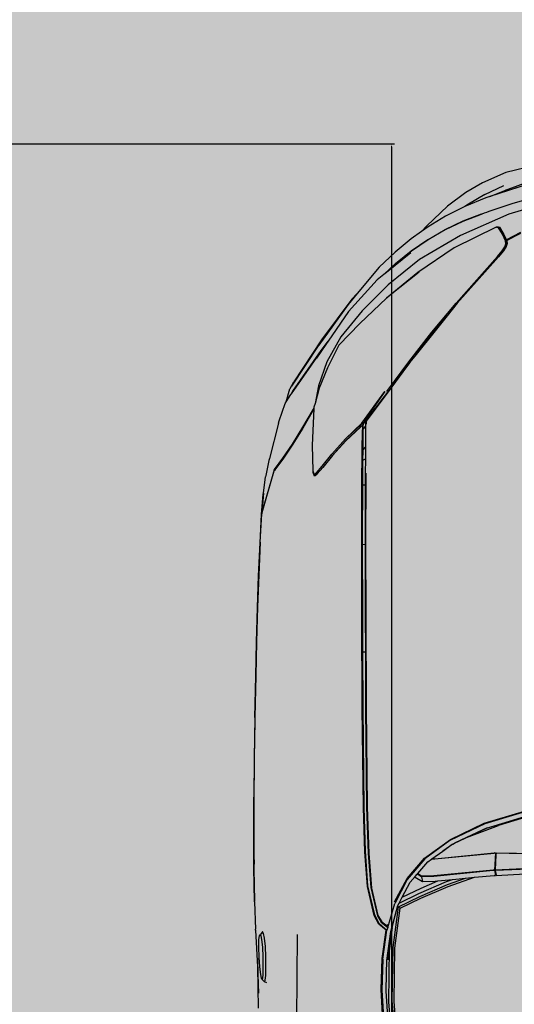
# Model space of a CAD drawing. Units: inches. Extents: x 1884 to 2398, y 474 to 1488.
# Tile 27 of 39: x 2275 to 2306, y 699 to 761. Entities that reach past the tile are written whole.
import ezdxf

# ---------------------------------------------------------------- set-up
doc = ezdxf.new("R2010")
doc.units = ezdxf.units.IN
doc.header["$MEASUREMENT"] = 0
doc.layers.get('0').update_dxf_attribs({"color": 250})
doc.layers.add('A-ANNO-DIMS', color=2, linetype='Continuous', lineweight=18)
doc.layers.add('C-VEHI', color=8, linetype='Continuous', lineweight=18)
doc.layers.add('Edges', color=250, linetype='Continuous')
doc.layers.add('L-PVMT-PATT', color=9, linetype='Continuous', lineweight=13, true_color=0xc7c8ca)
doc.styles.get("Standard").update_dxf_attribs({"font": 'arial.ttf'})
doc.dimstyles.get("Standard").update_dxf_attribs({"dimtxt": 7, "dimasz": 0.18, "dimexe": 0.18, "dimexo": 0.0625, "dimgap": 0.09, "dimtad": 0, "dimtih": 1, "dimtoh": 1, "dimzin": 0, "dimdsep": 46, "dimlunit": 3, "dimtxsty": 'Standard', "dimcen": 0.09, "dimadec": 0, "dimazin": 0, "dimtfac": 1, "dimtofl": 0, "dimtmove": 0, "dimatfit": 3, "dimfxl": 1, "dimtolj": 1, "dimtzin": 0, "dimarcsym": 0})

# ---------------------------------------------------------------- blocks, each defined once
blk = doc.blocks.new('Nissan Qashqai pl')
at = {"layer": 'Edges'}
for p, q in [((8.4086, 11.6764), (8.4045, 11.4011)), ((8.4305, 11.3996), (8.419, 11.6758)), ((8.4204, 11.6758), (8.4319, 11.3996)), ((8.4394, 11.4014), (8.4238, 11.6766)), ((7.3676, 11.5172), (7.3963, 11.4215)), ((7.3193, 11.4645), (7.3309, 11.4166)), ((8.3573, 11.3824), (8.3296, 11.4739)), ((8.3311, 11.4733), (8.3582, 11.3836)), ((8.3648, 11.3863), (8.3377, 11.4753)), ((8.3392, 11.4758), (8.3608, 11.4048)), ((7.344, 11.4572), (7.3596, 11.4139)), ((7.3467, 11.4596), (7.3686, 11.3913)), ((7.3489, 11.4517), (7.3686, 11.3913)), ((7.375, 11.4442), (7.3799, 11.4278)), ((7.4255, 11.4398), (7.4367, 11.4174)), ((7.4379, 11.4179), (7.4267, 11.4401)), ((8.4041, 11.4013), (8.4048, 11.4423)), ((7.3309, 11.4166), (7.347, 11.3798)), ((7.3799, 11.4278), (7.3845, 11.4136)), ((7.3963, 11.4215), (7.4302, 11.3449)), ((7.4387, 11.4162), (7.4282, 11.4113)), ((7.4283, 11.4135), (7.4359, 11.417)), ((7.4296, 11.4129), (7.4383, 11.417)), ((7.4359, 11.417), (7.4367, 11.4174)), ((7.4383, 11.417), (7.4367, 11.4174)), ((7.4375, 11.42), (7.4384, 11.4182)), ((7.4379, 11.4179), (7.4384, 11.4182)), ((7.4389, 11.4173), (7.4379, 11.4179)), ((7.4383, 11.417), (7.4379, 11.4179)), ((7.4389, 11.4173), (7.4383, 11.417)), ((7.4384, 11.4182), (7.4387, 11.4183)), ((7.4387, 11.4183), (7.443, 11.4188)), ((7.4431, 11.4166), (7.4387, 11.4162)), ((7.4389, 11.4173), (7.44, 11.4178)), ((7.4442, 11.4183), (7.44, 11.4178)), ((7.443, 11.4188), (7.4477, 11.4172)), ((7.4479, 11.4149), (7.4431, 11.4166)), ((7.4477, 11.4172), (7.4442, 11.4183)), ((7.4477, 11.4172), (7.4541, 11.4128)), ((7.3655, 11.3837), (7.3514, 11.4133)), ((7.3686, 11.3913), (7.3596, 11.4139)), ((7.3845, 11.4136), (7.3925, 11.3899)), ((7.4167, 11.4049), (7.417, 11.4065)), ((7.4172, 11.4047), (7.4167, 11.4049)), ((7.4169, 11.4036), (7.4167, 11.4049)), ((7.4282, 11.4113), (7.4169, 11.4044)), ((7.4172, 11.4047), (7.4169, 11.4044)), ((7.4169, 11.4044), (7.4169, 11.4036)), ((7.4172, 11.4018), (7.4169, 11.4036)), ((7.4169, 11.4036), (7.4169, 11.403)), ((7.4169, 11.403), (7.4172, 11.4011)), ((7.417, 11.4065), (7.4283, 11.4135)), ((7.4183, 11.406), (7.4172, 11.4047)), ((7.4174, 11.4013), (7.4172, 11.4018)), ((7.4172, 11.4011), (7.4498, 11.3349)), ((7.4174, 11.4013), (7.4175, 11.4012)), ((7.4296, 11.4129), (7.4183, 11.406)), ((7.4541, 11.4108), (7.4479, 11.4149)), ((7.4541, 11.4128), (7.4638, 11.4051)), ((7.4635, 11.4034), (7.4541, 11.4108)), ((7.5369, 11.3385), (7.4635, 11.4034)), ((7.4638, 11.4051), (7.5371, 11.34)), ((8.3799, 11.3545), (8.3608, 11.4048)), ((8.407, 11.401), (8.4037, 11.4002)), ((8.4037, 11.4002), (8.4314, 11.3985)), ((8.4037, 11.3992), (8.4037, 11.4002)), ((8.4041, 11.4013), (8.4045, 11.4011)), ((8.4045, 11.4011), (8.407, 11.401)), ((8.407, 11.401), (8.4305, 11.3996)), ((8.4314, 11.3985), (8.4394, 11.4004)), ((8.4319, 11.3996), (8.436, 11.4006)), ((8.436, 11.4006), (8.4394, 11.4014)), ((8.4394, 11.4004), (8.436, 11.4006)), ((8.4394, 11.3984), (8.4394, 11.4004)), ((7.3686, 11.3913), (7.3707, 11.3849)), ((7.3707, 11.3849), (7.3843, 11.3522)), ((7.3925, 11.3899), (7.3938, 11.3859)), ((7.3938, 11.3859), (7.3951, 11.3822)), ((8.3646, 11.387), (8.3799, 11.3545)), ((8.3888, 11.3355), (8.3648, 11.3863)), ((8.4037, 11.3992), (8.4046, 11.3981)), ((8.4042, 11.3983), (8.4037, 11.3992)), ((8.4134, 11.3049), (8.4042, 11.3983)), ((8.4046, 11.3981), (8.4138, 11.3048)), ((8.4305, 11.3996), (8.4319, 11.3996)), ((8.4306, 11.3966), (8.4314, 11.3975)), ((8.4398, 11.3032), (8.4306, 11.3966)), ((8.4314, 11.3985), (8.4314, 11.3975)), ((8.4314, 11.3975), (8.4319, 11.3967)), ((8.4319, 11.3967), (8.4412, 11.3033)), ((8.4425, 11.3672), (8.4394, 11.3984)), ((7.347, 11.3798), (7.3624, 11.3535)), ((7.3655, 11.3837), (7.3805, 11.3576)), ((7.3951, 11.3822), (7.3965, 11.3787)), ((7.3962, 11.3781), (7.3965, 11.3787)), ((7.4071, 11.3493), (7.3962, 11.3781)), ((7.3965, 11.3787), (7.3969, 11.3777)), ((7.3969, 11.3777), (7.4078, 11.349)), ((8.3826, 11.3291), (8.3573, 11.3824)), ((8.3582, 11.3836), (8.3844, 11.3284)), ((7.3624, 11.3535), (7.3837, 11.3245)), ((7.3805, 11.3576), (7.3843, 11.3522)), ((8.3799, 11.3545), (8.3888, 11.3355)), ((8.4571, 11.3258), (8.4425, 11.3672)), ((8.4439, 11.3531), (8.4425, 11.3672)), ((8.454, 11.3245), (8.4439, 11.3531)), ((8.4459, 11.3326), (8.4439, 11.3531)), ((7.3843, 11.3522), (7.3845, 11.3517)), ((7.3845, 11.3517), (7.3997, 11.3215)), ((7.4205, 11.3212), (7.4071, 11.3493)), ((7.4078, 11.349), (7.4211, 11.321)), ((7.4302, 11.3449), (7.4679, 11.2807)), ((7.5827, 11.3001), (7.5369, 11.3385)), ((7.5371, 11.34), (7.5568, 11.324)), ((7.3837, 11.3245), (7.4147, 11.2918)), ((7.4498, 11.3349), (7.4884, 11.2778)), ((7.584, 11.3013), (7.5568, 11.324)), ((7.5568, 11.324), (7.5829, 11.303)), ((8.4122, 11.2883), (8.3826, 11.3291)), ((8.3844, 11.3284), (8.4134, 11.2888)), ((8.3901, 11.3328), (8.3888, 11.3355)), ((8.3901, 11.3328), (8.4011, 11.3173)), ((8.3904, 11.3321), (8.3901, 11.3328)), ((8.4011, 11.3173), (8.3904, 11.3321)), ((8.4493, 11.3229), (8.4459, 11.3326)), ((8.4482, 11.3095), (8.4459, 11.3326)), ((8.468, 11.2793), (8.4493, 11.3229)), ((8.4725, 11.2812), (8.454, 11.3245)), ((8.4756, 11.2826), (8.4571, 11.3258)), ((7.3997, 11.3215), (7.4166, 11.2939)), ((7.4363, 11.294), (7.4205, 11.3212)), ((7.4211, 11.321), (7.4369, 11.2938)), ((8.4135, 11.3), (8.4011, 11.3173)), ((8.4594, 11.2831), (8.4482, 11.3095)), ((8.4487, 11.305), (8.4482, 11.3095)), ((7.4147, 11.2918), (7.4239, 11.2837)), ((7.4166, 11.2939), (7.4239, 11.2837)), ((7.4542, 11.2677), (7.4363, 11.294)), ((7.4369, 11.2938), (7.4549, 11.2675)), ((7.6296, 11.2639), (7.5827, 11.3001)), ((7.5829, 11.303), (7.618, 11.275)), ((7.618, 11.275), (7.584, 11.3013)), ((8.4135, 11.3), (8.4134, 11.3049)), ((8.4139, 11.2994), (8.4135, 11.3)), ((8.4138, 11.3048), (8.4139, 11.2994)), ((8.4183, 11.2934), (8.4139, 11.2994)), ((8.4365, 11.2776), (8.4183, 11.2934)), ((8.44, 11.2834), (8.4398, 11.3032)), ((8.4412, 11.3033), (8.4415, 11.2835)), ((8.4489, 11.2852), (8.4487, 11.305)), ((7.4239, 11.2837), (7.4354, 11.2675)), ((7.4679, 11.2807), (7.5081, 11.2311)), ((7.4882, 11.2797), (7.5243, 11.2341)), ((7.4884, 11.2778), (7.5289, 11.2283)), ((8.4444, 11.2608), (8.4122, 11.2883)), ((8.4134, 11.2888), (8.4462, 11.2609)), ((8.4365, 11.2776), (8.44, 11.2834)), ((8.4375, 11.2767), (8.4365, 11.2776)), ((8.4415, 11.2835), (8.4375, 11.2767)), ((8.4412, 11.2735), (8.4375, 11.2767)), ((8.4415, 11.2835), (8.4489, 11.2852)), ((8.4422, 11.2737), (8.4489, 11.2852)), ((8.4737, 11.2534), (8.4594, 11.2831)), ((8.4831, 11.2484), (8.468, 11.2793)), ((8.4889, 11.2473), (8.4725, 11.2812)), ((8.4914, 11.25), (8.4756, 11.2826)), ((7.4354, 11.2675), (7.4565, 11.2419)), ((7.4744, 11.2427), (7.4542, 11.2677)), ((7.4549, 11.2675), (7.475, 11.2426)), ((7.4574, 11.267), (7.4885, 11.2283)), ((7.618, 11.275), (7.6301, 11.2654)), ((7.676, 11.2289), (7.6296, 11.2639)), ((7.6301, 11.2654), (7.6306, 11.2651)), ((7.6306, 11.2651), (7.6306, 11.265)), ((7.6306, 11.265), (7.6373, 11.2601)), ((7.6373, 11.2601), (7.6769, 11.2312)), ((8.4422, 11.2737), (8.4412, 11.2735)), ((8.4499, 11.2659), (8.4412, 11.2735)), ((8.4814, 11.2413), (8.4444, 11.2608)), ((8.4462, 11.2609), (8.4838, 11.2415)), ((8.4737, 11.2534), (8.4499, 11.2659)), ((8.4831, 11.2484), (8.4737, 11.2534)), ((8.4867, 11.2465), (8.4831, 11.2484)), ((8.528, 11.2354), (8.4867, 11.2465)), ((8.5214, 11.2374), (8.4867, 11.2465)), ((8.4889, 11.2473), (8.4914, 11.25)), ((8.5531, 11.2387), (8.4889, 11.2473)), ((8.5544, 11.2416), (8.4914, 11.25)), ((8.7481, 11.2473), (8.6375, 11.2376)), ((8.7491, 11.2501), (8.6386, 11.2404)), ((7.4565, 11.2419), (7.4801, 11.2168)), ((7.4918, 11.2242), (7.4744, 11.2427)), ((7.475, 11.2426), (7.477, 11.2404)), ((7.477, 11.2404), (7.4765, 11.2411)), ((7.477, 11.2405), (7.4775, 11.2399)), ((7.4784, 11.2388), (7.477, 11.2404)), ((7.477, 11.2404), (7.4775, 11.2399)), ((7.4775, 11.2399), (7.4787, 11.2385)), ((7.4775, 11.2399), (7.4787, 11.2387)), ((7.4787, 11.2387), (7.4782, 11.2392)), ((7.4795, 11.2377), (7.4787, 11.2387)), ((7.4787, 11.2387), (7.4885, 11.2283)), ((7.5081, 11.2311), (7.5492, 11.1902)), ((7.5243, 11.2341), (7.5286, 11.2296)), ((7.6769, 11.2312), (7.7194, 11.1992)), ((7.7232, 11.1955), (7.6771, 11.2307)), ((8.5216, 11.2303), (8.4838, 11.2415)), ((8.5132, 11.2202), (8.5216, 11.2303)), ((8.5155, 11.2168), (8.5258, 11.2291)), ((8.5197, 11.2297), (8.5166, 11.2307)), ((8.5177, 11.2272), (8.5197, 11.2297)), ((8.5216, 11.2303), (8.5197, 11.2297)), ((8.5214, 11.2374), (8.555, 11.233)), ((8.5301, 11.2352), (8.5214, 11.2374)), ((8.5216, 11.2303), (8.5258, 11.2291)), ((8.5258, 11.2291), (8.5259, 11.2279)), ((8.5715, 11.2227), (8.5258, 11.2291)), ((8.5736, 11.2291), (8.528, 11.2354)), ((8.6375, 11.2376), (8.5531, 11.2387)), ((8.6386, 11.2404), (8.5544, 11.2416)), ((8.6387, 11.2319), (8.555, 11.233)), ((8.555, 11.233), (8.5726, 11.2307)), ((8.5941, 11.2286), (8.5736, 11.2291)), ((8.5941, 11.2289), (8.5941, 11.2286)), ((8.6699, 11.231), (8.622, 11.228)), ((8.6721, 11.2348), (8.6387, 11.2319)), ((7.4801, 11.2168), (7.5217, 11.1823)), ((7.4885, 11.2283), (7.4918, 11.2242)), ((7.4918, 11.2242), (7.5001, 11.2139)), ((7.5001, 11.2139), (7.5501, 11.1684)), ((7.5289, 11.2283), (7.5687, 11.1862)), ((7.7261, 11.1898), (7.6762, 11.2256)), ((7.6762, 11.2256), (7.7233, 11.1928)), ((8.4588, 11.2036), (8.5032, 11.2141)), ((8.4595, 11.2047), (8.5025, 11.2148)), ((8.5155, 11.2168), (8.5018, 11.2098)), ((8.5025, 11.2148), (8.5125, 11.221)), ((8.5163, 11.2162), (8.5029, 11.2092)), ((8.5032, 11.2141), (8.5132, 11.2202)), ((8.5125, 11.221), (8.5177, 11.2272)), ((8.5237, 11.2252), (8.5163, 11.2162)), ((8.5259, 11.2279), (8.5237, 11.2252)), ((8.5294, 11.2274), (8.5259, 11.2279)), ((8.5706, 11.2216), (8.5294, 11.2274)), ((8.6197, 11.2201), (8.5706, 11.2216)), ((8.5715, 11.2227), (8.6203, 11.2213)), ((8.622, 11.228), (8.5941, 11.2286)), ((8.6683, 11.2226), (8.6197, 11.2201)), ((8.6203, 11.2213), (8.6721, 11.2241)), ((7.7194, 11.1992), (7.7232, 11.1966)), ((8.1753, 11.1963), (8.3318, 11.198)), ((8.3318, 11.198), (8.4049, 11.2004)), ((8.332, 11.1971), (8.4042, 11.1995)), ((8.4559, 11.1991), (8.4014, 11.1953)), ((8.4571, 11.1983), (8.4022, 11.1943)), ((8.4042, 11.1995), (8.4588, 11.2036)), ((8.4049, 11.2004), (8.4595, 11.2047)), ((8.5018, 11.2098), (8.4559, 11.1991)), ((8.5029, 11.2092), (8.4571, 11.1983)), ((7.5304, 11.1737), (7.5217, 11.1823)), ((7.5217, 11.1823), (7.5387, 11.1682)), ((7.5492, 11.1902), (7.59, 11.1565)), ((7.5687, 11.1862), (7.6032, 11.1533)), ((7.7232, 11.1966), (7.7279, 11.1965)), ((7.7281, 11.1918), (7.7232, 11.1955)), ((7.7232, 11.1955), (7.7245, 11.1955)), ((7.7267, 11.1902), (7.7233, 11.1928)), ((7.7247, 11.1954), (7.7245, 11.1955)), ((7.7245, 11.1955), (7.7294, 11.1955)), ((7.7261, 11.1898), (7.7507, 11.1638)), ((7.7286, 11.1881), (7.7267, 11.1902)), ((7.7281, 11.1918), (7.7299, 11.1904)), ((7.7349, 11.1917), (7.7281, 11.1918)), ((7.753, 11.1648), (7.7281, 11.1918)), ((7.7507, 11.1638), (7.7286, 11.1881)), ((7.7294, 11.1955), (7.731, 11.1955)), ((7.7299, 11.1904), (7.7324, 11.1876)), ((7.7299, 11.1904), (7.7364, 11.1904)), ((7.731, 11.1955), (7.7349, 11.1917)), ((7.731, 11.1955), (7.764, 11.1953)), ((7.7324, 11.1876), (7.7539, 11.1642)), ((7.768, 11.1915), (7.7349, 11.1917)), ((7.7363, 11.1904), (7.7364, 11.1904)), ((7.7694, 11.1901), (7.7364, 11.1904)), ((7.764, 11.1953), (7.7636, 11.1957)), ((7.768, 11.1915), (7.764, 11.1953)), ((7.764, 11.1953), (7.7662, 11.1953)), ((7.7659, 11.1957), (7.7662, 11.1953)), ((7.7662, 11.1953), (7.7668, 11.1946)), ((7.7662, 11.1953), (7.7811, 11.1952)), ((7.7692, 11.1915), (7.768, 11.1915)), ((7.7694, 11.1901), (7.7687, 11.1908)), ((7.7844, 11.1913), (7.7692, 11.1915)), ((7.7707, 11.1901), (7.7694, 11.1901)), ((7.7851, 11.19), (7.7707, 11.1901)), ((7.7811, 11.1952), (7.7809, 11.1958)), ((7.7814, 11.1946), (7.7811, 11.1952)), ((7.7811, 11.1952), (7.7822, 11.1952)), ((7.7822, 11.1952), (7.7819, 11.1958)), ((7.7822, 11.1952), (7.8057, 11.195)), ((7.7844, 11.1913), (7.7822, 11.1952)), ((7.8078, 11.1911), (7.7844, 11.1913)), ((7.7846, 11.1909), (7.7851, 11.19)), ((7.8083, 11.1898), (7.7851, 11.19)), ((7.8048, 11.1959), (7.8233, 11.1958)), ((7.8057, 11.195), (7.8233, 11.195)), ((7.8233, 11.1911), (7.8078, 11.1911)), ((7.904, 11.1894), (7.8083, 11.1898)), ((7.8233, 11.195), (7.8233, 11.1958)), ((7.8233, 11.1958), (7.9014, 11.1955)), ((7.8233, 11.195), (7.902, 11.1947)), ((7.8233, 11.1911), (7.8233, 11.195)), ((7.8233, 11.1899), (7.8233, 11.1911)), ((7.9036, 11.1907), (7.8233, 11.1911)), ((7.9014, 11.1955), (7.9185, 11.1955)), ((7.902, 11.1947), (7.9183, 11.1947)), ((7.9176, 11.1908), (7.9036, 11.1907)), ((8.0276, 11.1896), (7.904, 11.1894)), ((7.9183, 11.1947), (7.9176, 11.1908)), ((8.0275, 11.1909), (7.9176, 11.1908)), ((7.9185, 11.1955), (7.9183, 11.1947)), ((7.9183, 11.1947), (8.0275, 11.1948)), ((7.9185, 11.1955), (8.0273, 11.1957)), ((8.0273, 11.1957), (8.1753, 11.1963)), ((8.0275, 11.1948), (8.0876, 11.1951)), ((8.0873, 11.1911), (8.0275, 11.1909)), ((8.1753, 11.1903), (8.0276, 11.1896)), ((8.0876, 11.1951), (8.0873, 11.1911)), ((8.1755, 11.1915), (8.0873, 11.1911)), ((8.0876, 11.1951), (8.1754, 11.1954)), ((8.3324, 11.192), (8.1753, 11.1903)), ((8.1754, 11.1954), (8.332, 11.1971)), ((8.3324, 11.1931), (8.1755, 11.1915)), ((8.4014, 11.1953), (8.3324, 11.1931)), ((8.4022, 11.1943), (8.3324, 11.192)), ((7.5304, 11.1737), (7.5946, 11.1262)), ((7.5387, 11.1682), (7.6031, 11.1217)), ((7.5501, 11.1684), (7.5969, 11.1365)), ((7.59, 11.1565), (7.6295, 11.1344)), ((7.6032, 11.1533), (7.6386, 11.1353)), ((7.7748, 11.1423), (7.7507, 11.1638)), ((7.753, 11.1648), (7.7772, 11.1431)), ((7.7539, 11.1642), (7.7772, 11.1431)), ((7.6113, 11.1256), (7.5969, 11.1365)), ((7.5969, 11.1365), (7.6021, 11.1329)), ((7.7938, 11.1271), (7.7748, 11.1423)), ((7.7772, 11.1431), (7.7959, 11.1281)), ((7.5946, 11.1262), (7.6608, 11.0825)), ((7.6021, 11.1329), (7.6118, 11.1255)), ((7.6021, 11.1329), (7.6237, 11.1181)), ((7.6676, 11.0791), (7.6024, 11.1221)), ((7.6759, 11.0809), (7.6113, 11.1256)), ((7.6118, 11.1255), (7.6799, 11.0783)), ((7.6295, 11.1344), (7.667, 11.1212)), ((7.6386, 11.1353), (7.6708, 11.1225)), ((7.667, 11.1212), (7.6949, 11.1158)), ((7.6708, 11.1225), (7.6949, 11.1158)), ((7.8045, 11.1179), (7.7938, 11.1271)), ((7.7959, 11.1281), (7.8062, 11.1192)), ((7.6949, 11.1158), (7.701, 11.1141)), ((7.701, 11.1141), (7.7024, 11.1141)), ((7.7038, 11.1132), (7.7024, 11.1141)), ((7.7024, 11.1141), (7.7034, 11.114)), ((7.7034, 11.114), (7.7056, 11.1128)), ((7.7034, 11.114), (7.7608, 11.1112)), ((7.7325, 11.0966), (7.7038, 11.1132)), ((7.7056, 11.1128), (7.7341, 11.0963)), ((7.7608, 11.1112), (7.8014, 11.1124)), ((7.8014, 11.1124), (7.8022, 11.1126)), ((7.8022, 11.1126), (7.8072, 11.1141)), ((7.8037, 11.1126), (7.8022, 11.1126)), ((7.8096, 11.1148), (7.8037, 11.1126)), ((7.8072, 11.1141), (7.8045, 11.1179)), ((7.8087, 11.1159), (7.8062, 11.1192)), ((7.8062, 11.1192), (7.8066, 11.1188)), ((7.8066, 11.1188), (7.8096, 11.1148)), ((7.8072, 11.1141), (7.8087, 11.1159)), ((7.7591, 11.08), (7.7325, 11.0966)), ((7.7341, 11.0963), (7.7606, 11.0798)), ((7.6712, 11.0767), (7.6608, 11.0825)), ((7.6721, 11.0762), (7.6712, 11.0767)), ((7.6926, 11.0705), (7.6721, 11.0762)), ((7.6793, 11.0784), (7.6759, 11.0809)), ((7.6802, 11.0782), (7.6793, 11.0784)), ((7.6802, 11.0782), (7.6799, 11.0783)), ((7.6809, 11.0777), (7.6802, 11.0782)), ((7.6926, 11.0705), (7.6809, 11.0777)), ((7.7814, 11.065), (7.7591, 11.08)), ((7.7606, 11.0798), (7.7828, 11.0649)), ((8.5326, 11.0874), (8.6675, 11.0866)), ((7.6953, 11.0688), (7.6926, 11.0705)), ((7.7223, 11.059), (7.6953, 11.0688)), ((7.7262, 11.0581), (7.7223, 11.059)), ((7.7262, 11.0581), (7.7819, 11.0438)), ((7.797, 11.0534), (7.7814, 11.065)), ((7.7828, 11.0649), (7.7984, 11.0533)), ((7.7819, 11.0438), (7.7848, 11.043)), ((7.7848, 11.043), (7.8087, 11.038)), ((7.797, 11.0534), (7.797, 11.0534)), ((7.7998, 11.0513), (7.797, 11.0534)), ((7.7984, 11.0533), (7.8007, 11.0516)), ((7.7998, 11.0513), (7.8676, 11.0318)), ((7.8007, 11.0516), (7.8002, 11.0517)), ((7.8007, 11.0516), (7.8012, 11.0513)), ((7.8681, 11.032), (7.8012, 11.0513)), ((7.8087, 11.038), (7.8106, 11.0377)), ((7.8107, 11.0377), (7.8106, 11.0377)), ((7.8363, 11.0344), (7.8107, 11.0377)), ((7.8381, 11.0342), (7.8363, 11.0344)), ((7.8363, 11.0344), (7.8676, 11.0318)), ((7.87, 11.0315), (7.8381, 11.0342)), ((7.8681, 11.032), (7.8676, 11.0318)), ((7.8681, 11.032), (7.869, 11.0317)), ((7.9137, 11.0292), (7.869, 11.0317)), ((7.9151, 11.029), (7.87, 11.0315)), ((7.9137, 11.0292), (7.9658, 11.027)), ((7.9668, 11.0268), (7.9151, 11.029)), ((7.9658, 11.027), (8.016, 11.0253)), ((8.5283, 11.0336), (8.5287, 11.0329)), ((8.531, 11.0346), (8.5287, 11.0329)), ((8.5287, 11.0329), (8.5331, 11.0292)), ((8.5385, 11.0363), (8.531, 11.0346)), ((8.5331, 11.0292), (8.5346, 11.0303)), ((8.5347, 11.0282), (8.5331, 11.0292)), ((8.5346, 11.0303), (8.5406, 11.0316)), ((8.5407, 11.0274), (8.5347, 11.0282)), ((8.5518, 11.0375), (8.5385, 11.0363)), ((8.5406, 11.0316), (8.5526, 11.0328)), ((8.5527, 11.0273), (8.5407, 11.0274)), ((8.568, 11.0382), (8.5518, 11.0375)), ((8.5526, 11.0328), (8.5681, 11.0335)), ((8.5682, 11.0278), (8.5527, 11.0273)), ((8.5842, 11.0384), (8.568, 11.0382)), ((8.5681, 11.0335), (8.5836, 11.0337)), ((8.5837, 11.0288), (8.5682, 11.0278)), ((8.5836, 11.0337), (8.5957, 11.0334)), ((8.5958, 11.0301), (8.5837, 11.0288)), ((8.5974, 11.0381), (8.5842, 11.0384)), ((8.5957, 11.0334), (8.6017, 11.0328)), ((8.6018, 11.0312), (8.5958, 11.0301)), ((8.6049, 11.0373), (8.5974, 11.0381)), ((8.6017, 11.0328), (8.6032, 11.0321)), ((8.6032, 11.0321), (8.6018, 11.0312)), ((8.6073, 11.0362), (8.6032, 11.0321)), ((8.6073, 11.0362), (8.6049, 11.0373)), ((8.609, 11.0397), (8.6073, 11.0362)), ((8.0168, 11.0251), (7.9668, 11.0268)), ((8.016, 11.0253), (8.0713, 11.0237)), ((8.0718, 11.0235), (8.0168, 11.0251)), ((8.0713, 11.0237), (8.1249, 11.0223)), ((8.1251, 11.0222), (8.0718, 11.0235)), ((8.1249, 11.0223), (8.1901, 11.021)), ((8.1902, 11.0208), (8.1251, 11.0222)), ((8.1901, 11.021), (8.1938, 11.021)), ((8.1902, 11.021), (8.1938, 11.021)), ((8.1904, 11.0209), (8.1902, 11.0208)), ((8.1904, 11.0209), (8.2543, 11.0198)), ((8.1938, 11.021), (8.1954, 11.0209)), ((8.1954, 11.0209), (8.2544, 11.02)), ((8.2544, 11.0198), (8.2543, 11.0199)), ((8.2543, 11.0198), (8.2544, 11.0198)), ((8.2544, 11.02), (8.3166, 11.0193)), ((8.2544, 11.0198), (8.2556, 11.0198)), ((8.2556, 11.0198), (8.256, 11.0198)), ((8.256, 11.0198), (8.2561, 11.0198)), ((8.2561, 11.0198), (8.2693, 11.0197)), ((8.2693, 11.0197), (8.2694, 11.0197)), ((8.2694, 11.0197), (8.3098, 11.0192)), ((8.3098, 11.0192), (8.3163, 11.0192)), ((8.3663, 11.019), (8.3163, 11.0192)), ((8.3597, 11.019), (8.3163, 11.0192)), ((8.3166, 11.0193), (8.3764, 11.0191)), ((8.3602, 11.019), (8.3597, 11.019)), ((8.3608, 11.019), (8.3602, 11.019)), ((8.3663, 11.019), (8.3608, 11.019)), ((8.3663, 11.019), (8.3764, 11.0191)), ((8.3757, 11.019), (8.3663, 11.019)), ((8.4282, 11.0193), (8.3757, 11.019)), ((8.3764, 11.0191), (8.4069, 11.0192)), ((8.4069, 11.0192), (8.4219, 11.0196)), ((8.4069, 11.0192), (8.4292, 11.0193)), ((8.4799, 11.0202), (8.4282, 11.0193)), ((8.4292, 11.0193), (8.4799, 11.0202)), ((8.4811, 11.0203), (8.4799, 11.0202)), ((8.4811, 11.0203), (8.5241, 11.022)), ((8.5259, 11.0221), (8.5241, 11.022)), ((8.5259, 11.0221), (8.5838, 11.0251)), ((8.5707, 11.0248), (8.5965, 11.0258)), ((8.5838, 11.0251), (8.6489, 11.0263)), ((8.5838, 11.0251), (8.5965, 11.0258)), ((8.5965, 11.0258), (8.6252, 11.0268))]:
    blk.add_line(p, q, dxfattribs=at)
blk = doc.blocks.new('car')
blk.add_blockref('Nissan Qashqai pl', (-9.7433, -11.9151))
blk = doc.blocks.new('carr')
blk.add_blockref('car', (0.5124, -0.007))
blk = doc.blocks.new('*D23')
at = {"layer": 'A-ANNO-DIMS', "color": 0, "lineweight": -2, "transparency": 16777216}
for p, q in [((2272.304, 752.812), (2298.291, 752.812)), ((2298.111, 752.632), (2298.111, 670.29)), ((2298.111, 580.529), (2298.111, 662.871)), ((2272.304, 580.349), (2298.291, 580.349))]:
    blk.add_line(p, q, dxfattribs=at)
at = {"layer": 'A-ANNO-DIMS', "color": 0, "lineweight": 100, "transparency": 16777216}
for points in [[(2298.081, 752.632), (2298.141, 752.632), (2298.111, 752.812)], [(2298.081, 580.529), (2298.141, 580.529), (2298.111, 580.349)]]:
    blk.add_solid(points, dxfattribs=at)
at = {"layer": 'Defpoints', "color": 0, "lineweight": 100, "transparency": 16777216}
for p in [(2272.242, 752.812), (2272.242, 580.349), (2298.111, 580.349)]:
    blk.add_point(p, dxfattribs=at)
at = {"layer": 'A-ANNO-DIMS', "color": 0, "transparency": 16777216, "insert": (2298.111, 666.58), "char_height": 7, "attachment_point": 5}
blk.add_mtext('\\A1;CAR 14\'-4 1/2" TYP.', dxfattribs=at)

msp = doc.modelspace()

# ---------------------------------------------------------------- hatches: boundary and pattern name
at = {"layer": 'L-PVMT-PATT'}
h = msp.add_hatch(color=256, dxfattribs=at)
h.dxf.hatch_style = 1
h.paths.add_polyline_path([(2387.529, 769.966), (2351.529, 769.966), (2238.447, 769.966), (2238.447, 762.15), (2238.447, 754.445), (2126.529, 754.445), (2126.529, 676.183), (2134.868, 676.183), (2142.673, 676.183), (2142.673, 646.578), (2134.868, 646.578), (2126.529, 646.578), (2126.529, 640.17), (2387.529, 640.17)])
h.paths.add_polyline_path([(2387.529, 631.385), (2303.086, 631.385), (2303.086, 615.671), (2387.529, 615.671)])
h.paths.add_polyline_path([(2387.529, 640.17), (2126.529, 640.17), (2126.529, 631.385), (2387.529, 631.385)])
h.paths.add_polyline_path([(2393.529, 604.13), (2387.529, 604.13), (2387.529, 615.671), (2303.086, 615.671), (2303.086, 607.943), (2249.649, 607.943), (2126.529, 607.943), (2126.529, 533.885), (2393.529, 533.885)])
h.paths.add_polyline_path([(2257.825, 611.008), (2257.83, 611.337), (2257.915, 616.493), (2258.021, 621.805), (2258.146, 627.274), (2258.252, 631.385), (2126.529, 631.385), (2126.529, 611.008)])
h.paths.add_polyline_path([(2258.892, 611.285), (2258.888, 611.008), (2300.247, 611.008), (2300.247, 631.385), (2259.314, 631.385), (2259.206, 627.173), (2259.081, 621.72), (2258.976, 616.424)])

# ---------------------------------------------------------------- block references
at = {"layer": 'C-VEHI', "xscale": 39.37007874015748, "yscale": 39.37007874015748, "zscale": 39.37007874015748, "rotation": 270}
msp.add_blockref('carr', (2325.111, 676.232), dxfattribs=at)

# ---------------------------------------------------------------- dimensions: what is measured, and where the dimension line sits
at = {"layer": 'A-ANNO-DIMS'}
dim = msp.add_linear_dim(base=(2298.111, 580.349), p1=(2272.242, 752.812), p2=(2272.242, 580.349), angle=270, text='CAR <> TYP.', dimstyle='Standard', override={"dimdec": 1, "dimlfac": 1, "dimrnd": 0, "dimzin": 1, "dimdsep": 46, "dimlunit": 4, "dimfrac": 2}, dxfattribs=at)
dim.commit()
dim.dimension.update_dxf_attribs({"geometry": '*D23', "text_midpoint": (2298.111, 666.58)})

doc.saveas('drawing.dxf')
